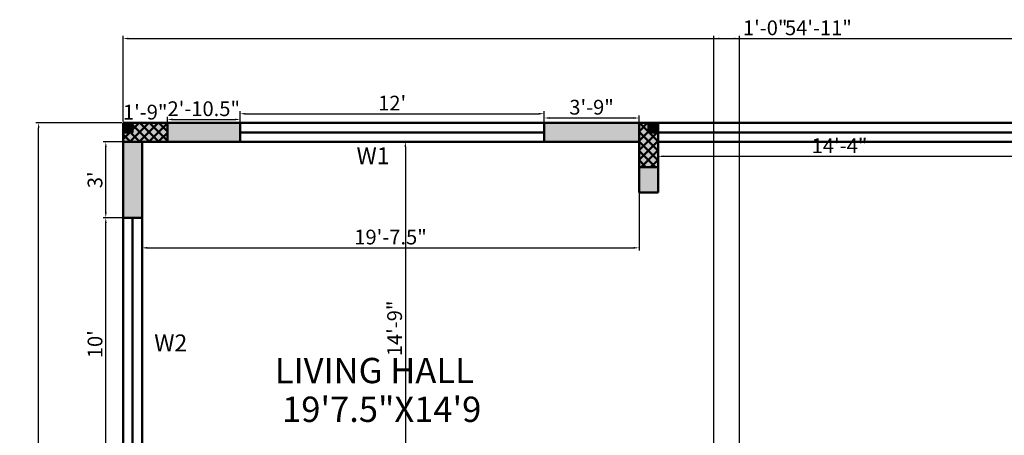
# Model space of a CAD drawing. Units: inches. Extents: x 1749 to 3550, y 1117 to 2383.
# Tile 3 of 15: x 1811 to 2277, y 1490 to 1687. Entities that reach past the tile are written whole.
import ezdxf

# ---------------------------------------------------------------- set-up
doc = ezdxf.new("R2010")
doc.units = ezdxf.units.IN
for name, color, linetype, lineweight in [('A-ANNO-DIMS', 2, 'Continuous', 18), ('A-ANNO-TEXT', 3, 'Continuous', 18), ('A-AREA-IDEN', 7, 'Continuous', 18), ('A-COLS', 10, 'Continuous', 50), ('A-WALL', 7, 'Continuous', 50), ('A-WALL-PATT', 8, 'Continuous', 13)]:
    doc.layers.add(name, color=color, linetype=linetype, lineweight=lineweight)
doc.styles.get("Standard").update_dxf_attribs({"font": 'arial.ttf'})
doc.dimstyles.new('ISO-25', dxfattribs={"dimtxt": 7, "dimasz": 2.5, "dimexe": 1.25, "dimexo": 0.625, "dimtad": 1, "dimdec": 1, "dimlunit": 3, "dimtxsty": 'Standard', "dimcen": 2.5, "dimadec": 0, "dimazin": 0, "dimtfac": 1, "dimtdec": 1, "dimtmove": 0, "dimatfit": 3, "dimfxl": 1, "dimarcsym": 0})

# ---------------------------------------------------------------- blocks, each defined once
blk = doc.blocks.new('*D15')
at = {"layer": 'A-ANNO-DIMS', "color": 0, "lineweight": -2, "ltscale": 0.5, "transparency": 16777216}
for p, q in [((1868.6, 1628.62), (1868.6, 1577.72)), ((2104.1, 1628.62), (2104.1, 1577.72)), ((1871.1, 1578.97), (2101.6, 1578.97))]:
    blk.add_line(p, q, dxfattribs=at)
at = {"layer": 'A-ANNO-DIMS', "color": 0, "ltscale": 0.5, "transparency": 16777216}
for points in [[(1871.1, 1579.39), (1871.1, 1578.56), (1868.6, 1578.97)], [(2101.6, 1579.39), (2101.6, 1578.56), (2104.1, 1578.97)]]:
    blk.add_solid(points, dxfattribs=at)
at = {"layer": 'Defpoints', "color": 0, "ltscale": 0.5, "transparency": 16777216}
for p in [(1868.6, 1629.24), (2104.1, 1629.24), (2104.1, 1578.97)]:
    blk.add_point(p, dxfattribs=at)
at = {"layer": 'A-ANNO-DIMS', "color": 0, "ltscale": 0.5, "transparency": 16777216, "insert": (1986.35, 1583.17), "char_height": 7, "attachment_point": 5}
blk.add_mtext('19\'-7.5"', dxfattribs=at)
blk = doc.blocks.new('*D16')
at = {"layer": 'A-ANNO-DIMS', "color": 0, "lineweight": -2, "ltscale": 0.5, "transparency": 16777216}
for p, q in [((1995.57, 1629.24), (1992.13, 1629.24)), ((1993.38, 1626.74), (1993.38, 1454.74)), ((1995.57, 1452.24), (1992.13, 1452.24))]:
    blk.add_line(p, q, dxfattribs=at)
at = {"layer": 'A-ANNO-DIMS', "color": 0, "ltscale": 0.5, "transparency": 16777216}
for points in [[(1992.96, 1626.74), (1993.8, 1626.74), (1993.38, 1629.24)], [(1992.96, 1454.74), (1993.8, 1454.74), (1993.38, 1452.24)]]:
    blk.add_solid(points, dxfattribs=at)
at = {"layer": 'Defpoints', "color": 0, "ltscale": 0.5, "transparency": 16777216}
for p in [(1996.2, 1629.24), (1993.38, 1452.24), (1996.2, 1452.24)]:
    blk.add_point(p, dxfattribs=at)
at = {"layer": 'A-ANNO-DIMS', "color": 0, "ltscale": 0.5, "transparency": 16777216, "insert": (1989.18, 1540.74), "char_height": 7, "attachment_point": 5, "rotation": 90}
blk.add_mtext('14\'-9"', dxfattribs=at)
blk = doc.blocks.new('*D32')
at = {"layer": 'A-ANNO-DIMS', "color": 0, "lineweight": -2, "ltscale": 0.5, "transparency": 16777216}
for p, q in [((1859.6, 1638.87), (1859.6, 1639.49)), ((1862.1, 1638.24), (1878.1, 1638.24)), ((1880.6, 1638.87), (1880.6, 1639.49))]:
    blk.add_line(p, q, dxfattribs=at)
at = {"layer": 'A-ANNO-DIMS', "color": 0, "ltscale": 0.5, "transparency": 16777216}
for points in [[(1862.1, 1638.66), (1862.1, 1637.83), (1859.6, 1638.24)], [(1878.1, 1638.66), (1878.1, 1637.83), (1880.6, 1638.24)]]:
    blk.add_solid(points, dxfattribs=at)
at = {"layer": 'Defpoints', "color": 0, "ltscale": 0.5, "transparency": 16777216}
for p in [(1859.6, 1638.24), (1880.6, 1638.24), (1880.6, 1638.24)]:
    blk.add_point(p, dxfattribs=at)
at = {"layer": 'A-ANNO-DIMS', "color": 0, "ltscale": 0.5, "transparency": 16777216, "insert": (1870.1, 1642.44), "char_height": 7, "attachment_point": 5}
blk.add_mtext('1\'-9"', dxfattribs=at)
blk = doc.blocks.new('*D33')
at = {"layer": 'A-ANNO-DIMS', "color": 0, "lineweight": -2, "ltscale": 0.5, "transparency": 16777216}
for p, q in [((1880.6, 1638.87), (1880.6, 1641.11)), ((1883.1, 1639.86), (1912.6, 1639.86)), ((1915.1, 1638.87), (1915.1, 1641.11))]:
    blk.add_line(p, q, dxfattribs=at)
at = {"layer": 'A-ANNO-DIMS', "color": 0, "ltscale": 0.5, "transparency": 16777216}
for points in [[(1883.1, 1640.28), (1883.1, 1639.44), (1880.6, 1639.86)], [(1912.6, 1640.28), (1912.6, 1639.44), (1915.1, 1639.86)]]:
    blk.add_solid(points, dxfattribs=at)
at = {"layer": 'Defpoints', "color": 0, "ltscale": 0.5, "transparency": 16777216}
for p in [(1880.6, 1638.24), (1915.1, 1639.86), (1915.1, 1638.24)]:
    blk.add_point(p, dxfattribs=at)
at = {"layer": 'A-ANNO-DIMS', "color": 0, "ltscale": 0.5, "transparency": 16777216, "insert": (1897.85, 1644.06), "char_height": 7, "attachment_point": 5}
blk.add_mtext('2\'-10.5"', dxfattribs=at)
blk = doc.blocks.new('*D34')
at = {"layer": 'A-ANNO-DIMS', "color": 0, "lineweight": -2, "ltscale": 0.5, "transparency": 16777216}
for p, q in [((1915.1, 1638.87), (1915.1, 1643.83)), ((1917.6, 1642.58), (2056.6, 1642.58)), ((2059.1, 1638.87), (2059.1, 1643.83))]:
    blk.add_line(p, q, dxfattribs=at)
at = {"layer": 'A-ANNO-DIMS', "color": 0, "ltscale": 0.5, "transparency": 16777216}
for points in [[(1917.6, 1643), (1917.6, 1642.17), (1915.1, 1642.58)], [(2056.6, 1643), (2056.6, 1642.17), (2059.1, 1642.58)]]:
    blk.add_solid(points, dxfattribs=at)
at = {"layer": 'Defpoints', "color": 0, "ltscale": 0.5, "transparency": 16777216}
for p in [(2059.1, 1642.58), (1915.1, 1638.24), (2059.1, 1638.24)]:
    blk.add_point(p, dxfattribs=at)
at = {"layer": 'A-ANNO-DIMS', "color": 0, "ltscale": 0.5, "transparency": 16777216, "insert": (1987.1, 1646.72), "char_height": 7, "attachment_point": 5}
blk.add_mtext("12'", dxfattribs=at)
blk = doc.blocks.new('*D35')
at = {"layer": 'A-ANNO-DIMS', "color": 0, "lineweight": -2, "ltscale": 0.5, "transparency": 16777216}
for p, q in [((2059.1, 1638.87), (2059.1, 1641.82)), ((2061.6, 1640.57), (2101.6, 1640.57)), ((2104.1, 1638.87), (2104.1, 1641.82))]:
    blk.add_line(p, q, dxfattribs=at)
at = {"layer": 'A-ANNO-DIMS', "color": 0, "ltscale": 0.5, "transparency": 16777216}
for points in [[(2061.6, 1640.98), (2061.6, 1640.15), (2059.1, 1640.57)], [(2101.6, 1640.98), (2101.6, 1640.15), (2104.1, 1640.57)]]:
    blk.add_solid(points, dxfattribs=at)
at = {"layer": 'Defpoints', "color": 0, "ltscale": 0.5, "transparency": 16777216}
for p in [(2059.1, 1638.24), (2104.1, 1640.57), (2104.1, 1638.24)]:
    blk.add_point(p, dxfattribs=at)
at = {"layer": 'A-ANNO-DIMS', "color": 0, "ltscale": 0.5, "transparency": 16777216, "insert": (2081.6, 1644.77), "char_height": 7, "attachment_point": 5}
blk.add_mtext('3\'-9"', dxfattribs=at)
blk = doc.blocks.new('*D36')
at = {"layer": 'A-ANNO-DIMS', "color": 0, "lineweight": -2, "ltscale": 0.5, "transparency": 16777216}
for p, q in [((2113.1, 1628.62), (2113.1, 1621.13)), ((2285.1, 1628.62), (2285.1, 1621.13)), ((2115.6, 1622.38), (2282.6, 1622.38))]:
    blk.add_line(p, q, dxfattribs=at)
at = {"layer": 'A-ANNO-DIMS', "color": 0, "ltscale": 0.5, "transparency": 16777216}
for points in [[(2115.6, 1622.8), (2115.6, 1621.97), (2113.1, 1622.38)], [(2282.6, 1622.8), (2282.6, 1621.97), (2285.1, 1622.38)]]:
    blk.add_solid(points, dxfattribs=at)
at = {"layer": 'Defpoints', "color": 0, "ltscale": 0.5, "transparency": 16777216}
for p in [(2113.1, 1629.24), (2285.1, 1629.24), (2285.1, 1622.38)]:
    blk.add_point(p, dxfattribs=at)
at = {"layer": 'A-ANNO-DIMS', "color": 0, "ltscale": 0.5, "transparency": 16777216, "insert": (2199.1, 1626.52), "char_height": 7, "attachment_point": 5}
blk.add_mtext('14\'-4"', dxfattribs=at)
blk = doc.blocks.new('*D73')
at = {"layer": 'A-ANNO-DIMS', "color": 0, "lineweight": -2, "ltscale": 0.5, "transparency": 16777216}
for p, q in [((1858.98, 1593.24), (1850.18, 1593.24)), ((1851.43, 1475.74), (1851.43, 1590.74)), ((1858.98, 1473.24), (1850.18, 1473.24))]:
    blk.add_line(p, q, dxfattribs=at)
at = {"layer": 'A-ANNO-DIMS', "color": 0, "ltscale": 0.5, "transparency": 16777216}
for points in [[(1851.01, 1590.74), (1851.84, 1590.74), (1851.43, 1593.24)], [(1851.01, 1475.74), (1851.84, 1475.74), (1851.43, 1473.24)]]:
    blk.add_solid(points, dxfattribs=at)
at = {"layer": 'Defpoints', "color": 0, "ltscale": 0.5, "transparency": 16777216}
for p in [(1851.43, 1593.24), (1859.6, 1593.24), (1859.6, 1473.24)]:
    blk.add_point(p, dxfattribs=at)
at = {"layer": 'A-ANNO-DIMS', "color": 0, "ltscale": 0.5, "transparency": 16777216, "insert": (1847.23, 1533.24), "char_height": 7, "attachment_point": 5, "rotation": 90}
blk.add_mtext("10'", dxfattribs=at)
blk = doc.blocks.new('*D74')
at = {"layer": 'A-ANNO-DIMS', "color": 0, "lineweight": -2, "ltscale": 0.5, "transparency": 16777216}
for p, q in [((1858.98, 1629.24), (1850.18, 1629.24)), ((1851.43, 1595.74), (1851.43, 1626.74)), ((1858.98, 1593.24), (1850.18, 1593.24))]:
    blk.add_line(p, q, dxfattribs=at)
at = {"layer": 'A-ANNO-DIMS', "color": 0, "ltscale": 0.5, "transparency": 16777216}
for points in [[(1851.01, 1626.74), (1851.84, 1626.74), (1851.43, 1629.24)], [(1851.01, 1595.74), (1851.84, 1595.74), (1851.43, 1593.24)]]:
    blk.add_solid(points, dxfattribs=at)
at = {"layer": 'Defpoints', "color": 0, "ltscale": 0.5, "transparency": 16777216}
for p in [(1851.43, 1629.24), (1859.6, 1629.24), (1859.6, 1593.24)]:
    blk.add_point(p, dxfattribs=at)
at = {"layer": 'A-ANNO-DIMS', "color": 0, "ltscale": 0.5, "transparency": 16777216, "insert": (1847.23, 1611.24), "char_height": 7, "attachment_point": 5, "rotation": 90}
blk.add_mtext("3'", dxfattribs=at)
blk = doc.blocks.new('*D172')
at = {"layer": 'A-ANNO-DIMS', "color": 0, "lineweight": -2, "ltscale": 0.5, "transparency": 16777216}
for p, q in [((1859.6, 1638.87), (1859.6, 1679.49)), ((1862.1, 1678.24), (2516.1, 1678.24)), ((2518.6, 1638.87), (2518.6, 1679.49))]:
    blk.add_line(p, q, dxfattribs=at)
at = {"layer": 'A-ANNO-DIMS', "color": 0, "ltscale": 0.5, "transparency": 16777216}
for points in [[(1862.1, 1678.66), (1862.1, 1677.83), (1859.6, 1678.24)], [(2516.1, 1678.66), (2516.1, 1677.83), (2518.6, 1678.24)]]:
    blk.add_solid(points, dxfattribs=at)
at = {"layer": 'Defpoints', "color": 0, "ltscale": 0.5, "transparency": 16777216}
for p in [(2518.6, 1678.24), (1859.6, 1638.24), (2518.6, 1638.24)]:
    blk.add_point(p, dxfattribs=at)
at = {"layer": 'A-ANNO-DIMS', "color": 0, "ltscale": 0.5, "transparency": 16777216, "insert": (2189.1, 1682.44), "char_height": 7, "attachment_point": 5}
blk.add_mtext('54\'-11"', dxfattribs=at)
blk = doc.blocks.new('*D173')
at = {"layer": 'A-ANNO-DIMS', "color": 0, "lineweight": -2, "ltscale": 0.5, "transparency": 16777216}
for p, q in [((1858.98, 1638.24), (1818.35, 1638.24)), ((1819.6, 1212.74), (1819.6, 1635.74)), ((1858.98, 1210.24), (1818.35, 1210.24))]:
    blk.add_line(p, q, dxfattribs=at)
at = {"layer": 'A-ANNO-DIMS', "color": 0, "ltscale": 0.5, "transparency": 16777216}
for points in [[(1819.19, 1635.74), (1820.02, 1635.74), (1819.6, 1638.24)], [(1819.19, 1212.74), (1820.02, 1212.74), (1819.6, 1210.24)]]:
    blk.add_solid(points, dxfattribs=at)
at = {"layer": 'Defpoints', "color": 0, "ltscale": 0.5, "transparency": 16777216}
for p in [(1819.6, 1638.24), (1859.6, 1638.24), (1859.6, 1210.24)]:
    blk.add_point(p, dxfattribs=at)
at = {"layer": 'A-ANNO-DIMS', "color": 0, "ltscale": 0.5, "transparency": 16777216, "insert": (1815.4, 1424.24), "char_height": 7, "attachment_point": 5, "rotation": 90}
blk.add_mtext('35\'-8"', dxfattribs=at)
blk = doc.blocks.new('*D177')
at = {"layer": 'A-ANNO-DIMS', "color": 0, "lineweight": -2, "ltscale": 0.5, "transparency": 16777216}
for p, q in [((2139.6, 1319.37), (2139.6, 1679.49)), ((2142.1, 1678.24), (2149.27, 1678.24)), ((2151.77, 1319.37), (2151.77, 1679.49)), ((2151.77, 1678.24), (2173.47, 1678.24))]:
    blk.add_line(p, q, dxfattribs=at)
at = {"layer": 'A-ANNO-DIMS', "color": 0, "ltscale": 0.5, "transparency": 16777216}
for points in [[(2142.1, 1678.66), (2142.1, 1677.83), (2139.6, 1678.24)], [(2149.27, 1678.66), (2149.27, 1677.83), (2151.77, 1678.24)]]:
    blk.add_solid(points, dxfattribs=at)
at = {"layer": 'Defpoints', "color": 0, "ltscale": 0.5, "transparency": 16777216}
for p in [(2151.77, 1678.24), (2139.6, 1318.74), (2151.77, 1318.74)]:
    blk.add_point(p, dxfattribs=at)
at = {"layer": 'A-ANNO-DIMS', "color": 0, "ltscale": 0.5, "transparency": 16777216, "insert": (2163.87, 1682.44), "char_height": 7, "attachment_point": 5}
blk.add_mtext('1\'-0"', dxfattribs=at)

msp = doc.modelspace()

# ---------------------------------------------------------------- hatches: boundary and pattern name
at = {"layer": 'A-COLS', "ltscale": 10}
h = msp.add_hatch(color=256, dxfattribs=at)
h.dxf.hatch_style = 1
h.paths.add_polyline_path([(1859.6, 1638.24), (1859.6, 1633.74), (1864.1, 1633.74), (1864.1, 1638.24)])
h = msp.add_hatch(dxfattribs=at)
h.set_pattern_fill('ANSI37', color=256)
h.set_pattern_definition([(45, (208.36, 271.1368), (-2.245064, 2.245064), []), (135, (208.36, 271.1368), (-2.245064, -2.245064), [])])
h.paths.add_polyline_path([(1880.6, 1629.24), (1880.6, 1638.24), (1859.6, 1638.24), (1859.6, 1629.24)])
h = msp.add_hatch(dxfattribs=at)
h.set_pattern_fill('ANSI37', color=256, angle=90)
h.set_pattern_definition([(135, (3471.2103, -34.0015), (-2.245064, -2.245064), []), (225, (3471.2103, -34.0015), (2.245064, -2.245064), [])])
h.paths.add_polyline_path([(2113.1, 1638.24), (2104.1, 1638.24), (2104.1, 1617.24), (2113.1, 1617.24)])
h = msp.add_hatch(color=256, dxfattribs=at)
h.dxf.hatch_style = 1
h.paths.add_polyline_path([(2108.6, 1638.24), (2108.6, 1633.74), (2113.1, 1633.74), (2113.1, 1638.24)])
at = {"layer": 'A-WALL-PATT', "ltscale": 10}
h = msp.add_hatch(color=256, dxfattribs=at)
h.dxf.hatch_style = 1
h.paths.add_polyline_path([(1915.1, 1629.24), (1915.1, 1638.24), (1859.6, 1638.24), (1859.6, 1593.24), (1868.6, 1593.24), (1868.6, 1629.24)])
h = msp.add_hatch(color=256, dxfattribs=at)
h.dxf.hatch_style = 1
h.paths.add_polyline_path([(2104.1, 1629.24), (2104.1, 1605.24), (2113.1, 1605.24), (2113.1, 1638.24), (2059.1, 1638.24), (2059.1, 1629.24)])

# ---------------------------------------------------------------- linework, layer by layer
at = {"layer": 'A-COLS', "ltscale": 10}
for points in [[(1859.6, 1638.24), (1864.1, 1638.24), (1864.1, 1633.74), (1859.6, 1633.74)], [(1859.6, 1638.24), (1880.6, 1638.24), (1880.6, 1629.24), (1859.6, 1629.24)], [(2104.1, 1617.24), (2104.1, 1638.24), (2113.1, 1638.24), (2113.1, 1617.24)], [(2108.6, 1638.24), (2113.1, 1638.24), (2113.1, 1633.74), (2108.6, 1633.74)]]:
    msp.add_lwpolyline(points, close=True, dxfattribs=at)
at = {"layer": 'A-WALL', "ltscale": 0.2}
for p, q in [((1859.6, 1638.24), (2518.6, 1638.24)), ((1859.6, 1638.24), (1859.6, 1210.24)), ((1915.1, 1629.24), (1915.1, 1638.24)), ((2059.1, 1629.24), (2059.1, 1638.24)), ((2113.1, 1638.24), (2113.1, 1605.24)), ((1915.1, 1633.74), (2059.1, 1633.74)), ((1868.6, 1629.24), (2104.1, 1629.24)), ((1868.6, 1629.24), (1868.6, 1452.24)), ((2104.1, 1629.24), (2104.1, 1605.24)), ((2113.1, 1629.24), (2285.1, 1629.24)), ((2113.1, 1605.24), (2104.1, 1605.24)), ((1868.6, 1593.24), (1859.6, 1593.24)), ((1864.1, 1593.24), (1864.1, 1473.24))]:
    msp.add_line(p, q, dxfattribs=at)
at = {"layer": 'A-WALL', "ltscale": 0.5}
msp.add_line((2285.1, 1633.74), (2113.1, 1633.74), dxfattribs=at)

# ---------------------------------------------------------------- texts
at = {"layer": 'A-ANNO-TEXT', "ltscale": 0.5}
for s, p in [('W1', (1970.24, 1618.63)), ('W2', (1874.39, 1529.87))]:
    msp.add_text(s, height=8, dxfattribs=at).set_placement(p)
at = {"layer": 'A-AREA-IDEN', "ltscale": 0.5}
msp.add_text('LIVING HALL ', height=12, rotation=0.0333, dxfattribs=at).set_placement((1931.51, 1514.72))
msp.add_text('19\'7.5"X14\'9', height=12, dxfattribs=at).set_placement((1934.97, 1496.37))

# ---------------------------------------------------------------- dimensions: what is measured, and where the dimension line sits
at = {"layer": 'A-ANNO-DIMS', "ltscale": 0.5}
for base, p1, p2, override, picture, middle in [((2518.6, 1678.24), (1859.6, 1638.24), (2518.6, 1638.24), {"dimdec": 1, "dimlfac": 1, "dimrnd": 0, "dimzin": 1, "dimdsep": 46, "dimlunit": 4, "dimfrac": 2}, '*D172', (2189.1, 1682.44)), ((2151.77, 1678.24), (2139.6, 1318.74), (2151.77, 1318.74), {"dimdec": 1, "dimlfac": 1, "dimrnd": 0, "dimzin": 1, "dimdsep": 46, "dimlunit": 4, "dimfrac": 2}, '*D177', (2163.87, 1682.44)), ((1880.6, 1638.24), (1859.6, 1638.24), (1880.6, 1638.24), {"dimclrd": 0, "dimclre": 0, "dimclrt": 0}, '*D32', (1870.1, 1642.44)), ((1915.1, 1639.86), (1880.6, 1638.24), (1915.1, 1638.24), {"dimclrd": 0, "dimclre": 0, "dimclrt": 0}, '*D33', (1897.85, 1644.06)), ((2059.1, 1642.58), (1915.1, 1638.24), (2059.1, 1638.24), {"dimclrd": 0, "dimclre": 0, "dimclrt": 0}, '*D34', (1987.1, 1646.72)), ((2104.1, 1640.57), (2059.1, 1638.24), (2104.1, 1638.24), {"dimclrd": 0, "dimclre": 0, "dimclrt": 0}, '*D35', (2081.6, 1644.77)), ((2104.1, 1578.97), (1868.6, 1629.24), (2104.1, 1629.24), {"dimclrd": 0, "dimclre": 0, "dimclrt": 0}, '*D15', (1986.35, 1583.17)), ((2285.1, 1622.38), (2113.1, 1629.24), (2285.1, 1629.24), {"dimclrd": 0, "dimclre": 0, "dimclrt": 0}, '*D36', (2199.1, 1626.52))]:
    dim = msp.add_linear_dim(base=base, p1=p1, p2=p2, dimstyle='ISO-25', override=override, dxfattribs=at)
    dim.commit()
    dim.dimension.update_dxf_attribs({"geometry": picture, "text_midpoint": middle})
for base, p1, p2, override, picture, middle in [((1819.6, 1638.24), (1859.6, 1210.24), (1859.6, 1638.24), {"dimdec": 1, "dimlfac": 1, "dimrnd": 0, "dimzin": 1, "dimdsep": 46, "dimlunit": 4, "dimfrac": 2}, '*D173', (1815.4, 1424.24)), ((1851.43, 1629.24), (1859.6, 1593.24), (1859.6, 1629.24), {"dimclrd": 0, "dimclre": 0, "dimclrt": 0}, '*D74', (1847.23, 1611.24)), ((1993.38, 1452.24), (1996.2, 1629.24), (1996.2, 1452.24), {"dimclrd": 0, "dimclre": 0, "dimclrt": 0}, '*D16', (1989.18, 1540.74)), ((1851.43, 1593.24), (1859.6, 1473.24), (1859.6, 1593.24), {"dimclrd": 0, "dimclre": 0, "dimclrt": 0}, '*D73', (1847.23, 1533.24))]:
    dim = msp.add_linear_dim(base=base, p1=p1, p2=p2, angle=90, dimstyle='ISO-25', override=override, dxfattribs=at)
    dim.commit()
    dim.dimension.update_dxf_attribs({"geometry": picture, "text_midpoint": middle})

doc.saveas('drawing.dxf')
